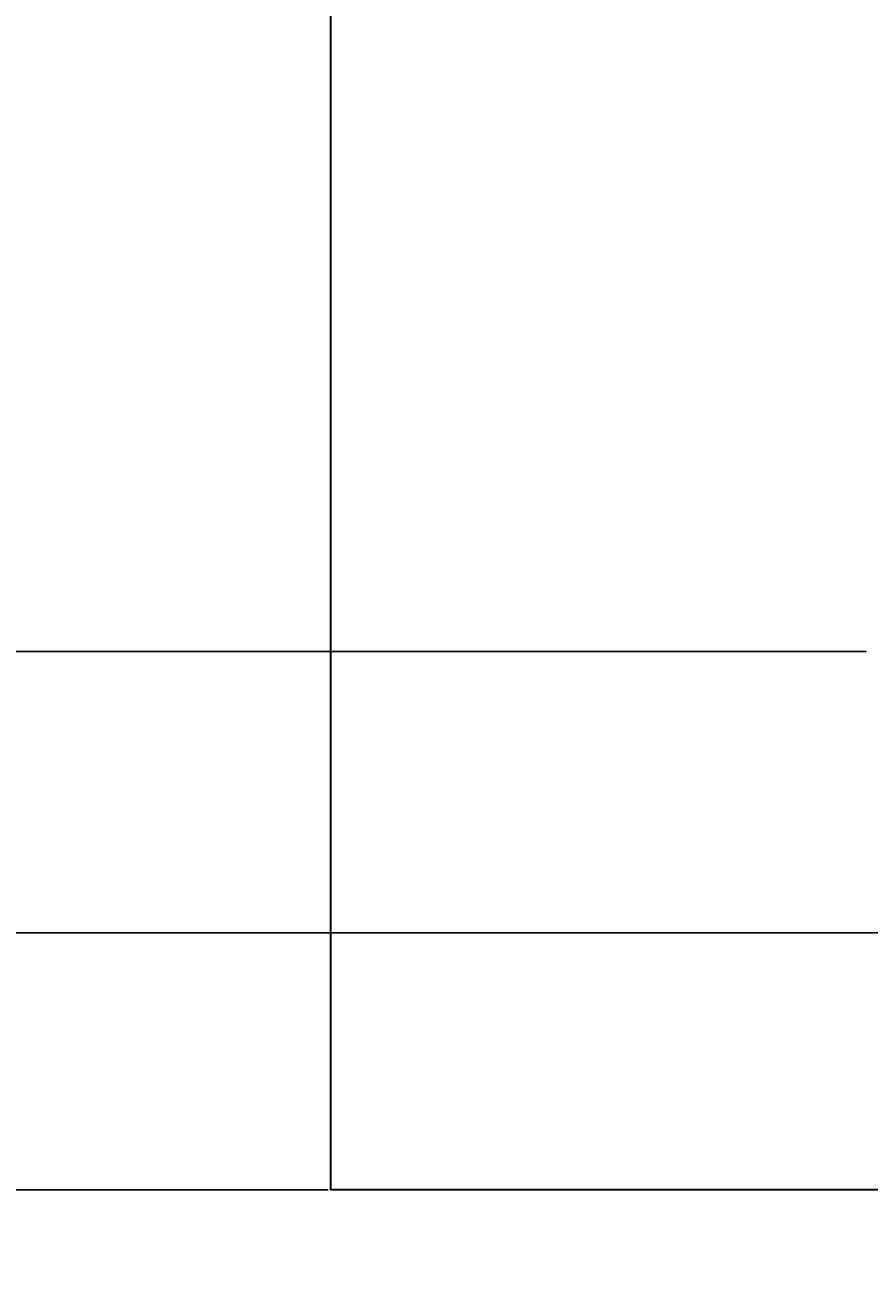
# Model space of a CAD drawing. Units: inches. Extents: x -6 to 289, y -8 to 323.
# Tile 11 of 107: x 27 to 46, y 68 to 96. Entities that reach past the tile are written whole.
import ezdxf

# ---------------------------------------------------------------- set-up
doc = ezdxf.new("R2010")
doc.units = ezdxf.units.IN
doc.header["$MEASUREMENT"] = 0
doc.layers.add('A-ANNO-DIMS', color=2, linetype='Continuous', lineweight=18)
doc.layers.add('A-ELEV', color=7, linetype='Continuous', lineweight=35)
doc.styles.get("Standard").update_dxf_attribs({"font": 'arial.ttf'})
doc.dimstyles.get("Standard").update_dxf_attribs({"dimtxt": 0.18, "dimasz": 0.18, "dimexe": 0.18, "dimexo": 0.0625, "dimgap": 0.09, "dimtad": 0, "dimtih": 1, "dimtoh": 1, "dimdec": 4, "dimzin": 0, "dimdsep": 46, "dimtxsty": 'Standard', "dimcen": 0.09, "dimadec": 0, "dimazin": 0, "dimtfac": 1, "dimtdec": 4, "dimtofl": 0, "dimtmove": 0, "dimatfit": 3, "dimfxl": 1, "dimtolj": 1, "dimtzin": 0, "dimarcsym": 0})

# ---------------------------------------------------------------- blocks, each defined once
blk = doc.blocks.new('*D17')
at = {"layer": 'A-ANNO-DIMS', "color": 0, "lineweight": -2, "transparency": 16777216}
for p, q in [((33.681, 70.243), (-5.737, 70.243)), ((-5.557, 70.063), (-5.557, 38.948)), ((-5.557, 7.469), (-5.557, 38.584)), ((11.907, 7.289), (-5.737, 7.289))]:
    blk.add_line(p, q, dxfattribs=at)
at = {"layer": 'A-ANNO-DIMS', "color": 0, "transparency": 16777216}
for points in [[(-5.587, 70.063), (-5.527, 70.063), (-5.557, 70.243)], [(-5.587, 7.469), (-5.527, 7.469), (-5.557, 7.289)]]:
    blk.add_solid(points, dxfattribs=at)
at = {"layer": 'Defpoints', "color": 0, "transparency": 16777216}
for p in [(-5.557, 70.243), (33.744, 70.243), (11.969, 7.289)]:
    blk.add_point(p, dxfattribs=at)
at = {"layer": 'A-ANNO-DIMS', "color": 0, "transparency": 16777216, "insert": (-5.557, 38.766), "char_height": 0.18, "attachment_point": 5}
blk.add_mtext('\\A1;62.95', dxfattribs=at)
blk = doc.blocks.new('*D18')
at = {"layer": 'A-ANNO-DIMS', "color": 0, "lineweight": -2, "transparency": 16777216}
for p, q in [((45.681, 82.243), (-5.737, 82.243)), ((-5.557, 82.063), (-5.557, 76.423)), ((-5.557, 70.423), (-5.557, 76.062)), ((33.681, 70.243), (-5.737, 70.243))]:
    blk.add_line(p, q, dxfattribs=at)
at = {"layer": 'A-ANNO-DIMS', "color": 0, "transparency": 16777216}
for points in [[(-5.587, 82.063), (-5.527, 82.063), (-5.557, 82.243)], [(-5.587, 70.423), (-5.527, 70.423), (-5.557, 70.243)]]:
    blk.add_solid(points, dxfattribs=at)
at = {"layer": 'Defpoints', "color": 0, "transparency": 16777216}
for p in [(-5.557, 82.243), (45.744, 82.243), (33.744, 70.243)]:
    blk.add_point(p, dxfattribs=at)
at = {"layer": 'A-ANNO-DIMS', "color": 0, "transparency": 16777216, "insert": (-5.557, 76.243), "char_height": 0.18, "attachment_point": 5}
blk.add_mtext('\\A1;12', dxfattribs=at)
blk = doc.blocks.new('*D19')
at = {"layer": 'A-ANNO-DIMS', "color": 0, "lineweight": -2, "transparency": 16777216}
for p, q in [((45.681, 277.043), (-5.737, 277.043)), ((-5.557, 276.863), (-5.557, 179.825)), ((-5.557, 82.423), (-5.557, 179.461)), ((45.681, 82.243), (-5.737, 82.243))]:
    blk.add_line(p, q, dxfattribs=at)
at = {"layer": 'A-ANNO-DIMS', "color": 0, "transparency": 16777216}
for points in [[(-5.587, 276.863), (-5.527, 276.863), (-5.557, 277.043)], [(-5.587, 82.423), (-5.527, 82.423), (-5.557, 82.243)]]:
    blk.add_solid(points, dxfattribs=at)
at = {"layer": 'Defpoints', "color": 0, "transparency": 16777216}
for p in [(-5.557, 277.043), (45.744, 277.043), (45.744, 82.243)]:
    blk.add_point(p, dxfattribs=at)
at = {"layer": 'A-ANNO-DIMS', "color": 0, "transparency": 16777216, "insert": (-5.557, 179.643), "char_height": 0.18, "attachment_point": 5}
blk.add_mtext('\\A1;194.8', dxfattribs=at)
blk = doc.blocks.new('*D86')
at = {"layer": 'A-ANNO-DIMS', "color": 0, "lineweight": -2, "transparency": 16777216}
for p, q in [((166.233, 75.971), (-5.737, 75.971)), ((-5.557, 75.791), (-5.557, 63.71)), ((-5.557, 51.265), (-5.557, 63.346)), ((120.945, 51.085), (-5.737, 51.085))]:
    blk.add_line(p, q, dxfattribs=at)
at = {"layer": 'A-ANNO-DIMS', "color": 0, "transparency": 16777216}
for points in [[(-5.587, 75.791), (-5.527, 75.791), (-5.557, 75.971)], [(-5.587, 51.265), (-5.527, 51.265), (-5.557, 51.085)]]:
    blk.add_solid(points, dxfattribs=at)
at = {"layer": 'Defpoints', "color": 0, "transparency": 16777216}
for p in [(-5.557, 75.971), (166.296, 75.971), (121.008, 51.085)]:
    blk.add_point(p, dxfattribs=at)
at = {"layer": 'A-ANNO-DIMS', "color": 0, "transparency": 16777216, "insert": (-5.557, 63.528), "char_height": 0.18, "attachment_point": 5}
blk.add_mtext('\\A1;24.886', dxfattribs=at)
blk = doc.blocks.new('*D87')
at = {"layer": 'A-ANNO-DIMS', "color": 0, "lineweight": -2, "transparency": 16777216}
for p, q in [((142.233, 108.948), (-5.737, 108.948)), ((-5.557, 108.768), (-5.557, 92.641)), ((-5.557, 76.151), (-5.557, 92.277)), ((166.233, 75.971), (-5.737, 75.971))]:
    blk.add_line(p, q, dxfattribs=at)
at = {"layer": 'A-ANNO-DIMS', "color": 0, "transparency": 16777216}
for points in [[(-5.587, 108.768), (-5.527, 108.768), (-5.557, 108.948)], [(-5.587, 76.151), (-5.527, 76.151), (-5.557, 75.971)]]:
    blk.add_solid(points, dxfattribs=at)
at = {"layer": 'Defpoints', "color": 0, "transparency": 16777216}
for p in [(-5.557, 108.948), (142.296, 108.948), (166.296, 75.971)]:
    blk.add_point(p, dxfattribs=at)
at = {"layer": 'A-ANNO-DIMS', "color": 0, "transparency": 16777216, "insert": (-5.557, 92.459), "char_height": 0.18, "attachment_point": 5}
blk.add_mtext('\\A1;32.98', dxfattribs=at)

msp = doc.modelspace()

# ---------------------------------------------------------------- linework, layer by layer
at = {"layer": 'A-ELEV'}
msp.add_lwpolyline([(33.7437, 289.0427), (99.7007, 289.0427), (99.7007, 70.2425), (33.7437, 70.2425)], close=True, dxfattribs=at)

# ---------------------------------------------------------------- dimensions: what is measured, and where the dimension line sits
at = {"layer": 'A-ANNO-DIMS'}
for base, p1, p2, override, picture, middle in [((-5.557, 277.0427), (45.7437, 82.2425), (45.7437, 277.0427), {"dimdec": 1, "dimlfac": 1, "dimrnd": 0, "dimzin": 0, "dimdsep": 46, "dimlunit": 2}, '*D19', (-5.557, 179.6426)), ((-5.557, 108.9477), (166.296, 75.9706), (142.296, 108.9477), {"dimdec": 2, "dimlfac": 1, "dimrnd": 0, "dimzin": 0, "dimdsep": 46, "dimlunit": 2}, '*D87', (-5.557, 92.4592)), ((-5.557, 82.2425), (33.7437, 70.2425), (45.7437, 82.2425), {"dimdec": 0, "dimlfac": 1, "dimrnd": 0, "dimzin": 0, "dimdsep": 46, "dimlunit": 2}, '*D18', (-5.557, 76.2425)), ((-5.557, 75.97064), (121.00798, 51.08513), (166.29599, 75.97064), {"dimdec": 3, "dimlfac": 1, "dimrnd": 0, "dimzin": 0, "dimdsep": 46, "dimlunit": 2}, '*D86', (-5.557, 63.52788)), ((-5.557, 70.2425), (11.9692, 7.2888), (33.7437, 70.2425), {"dimdec": 2, "dimlfac": 1, "dimrnd": 0, "dimzin": 0, "dimdsep": 46, "dimlunit": 2}, '*D17', (-5.557, 38.7657))]:
    dim = msp.add_linear_dim(base=base, p1=p1, p2=p2, angle=90, dimstyle='Standard', override=override, dxfattribs=at)
    dim.commit()
    dim.dimension.update_dxf_attribs({"geometry": picture, "text_midpoint": middle})

doc.saveas('drawing.dxf')
